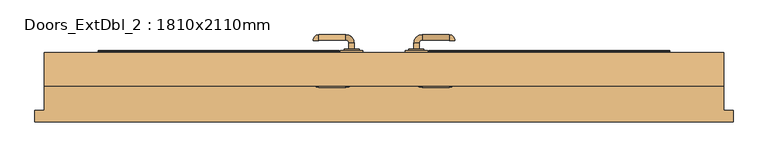
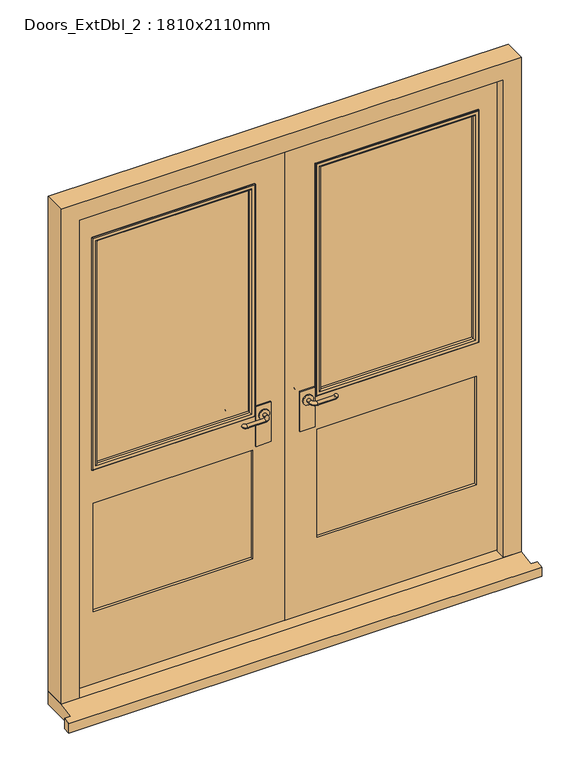
"""IFC4 building model written with IfcOpenShell, lengths in millimetres: door geometry, Doors_ExtDbl_2 : 1810x2110mm."""

from ifc_helpers import new_model, si_unit, point, frame, frame_2d, origin, place, context, project, spatial, polyline, circle_curve, ellipse_curve, trimmed, segment, composite_curve, outline, extrude, faceted_brep, source, transform, mapped, element, save
from ifc_brep_helpers import plane_surface, cylinder_surface, revolved_surface, advanced_brep


def doors_extdbl_2_1810x2110mm_9ab1935a(model_context):
    return source(origin(), model_context, "Body", "SolidModel", [
        extrude(outline(composite_curve([segment(trimmed(circle_curve(frame_2d((950.0, 86.5)), 20.0), [point((950.0, 66.5))], [point((950.0, 106.5))], False, "CARTESIAN"), True, "CONTINUOUS"), segment(trimmed(circle_curve(frame_2d((950.0, 86.5)), 20.0), [point((950.0, 106.5))], [point((950.0, 66.5))], False, "CARTESIAN"), True, "CONTINUOUS")], self_intersect=False)), frame((0.0, 58.4, 0.0), z_axis=(0.0, 1.0, 0.0), x_axis=(0.0, 0.0, 1.0)), (0.0, 0.0, 1.0), 4.5929895),
        advanced_brep(
        [(93.5, 62.9929895, 950.0), (79.5, 62.9929895, 950.0), (93.5, 78.4, 950.0), (79.5, 78.4, 950.0), (101.5, 100.4, 950.0), (101.5, 86.4, 950.0), (173.5, 86.4, 950.0), (173.5, 100.4, 950.0), (174.5, 85.4, 950.0), (188.5, 85.4, 950.0)],
        [
            (0, 1, circle_curve(frame((86.5, 62.9929895, 950.0), z_axis=(0.0, -1.0, 0.0), x_axis=(-1.0, 0.0, 0.0)), 7.0)),
            (1, 0, circle_curve(frame((86.5, 62.9929895, 950.0), z_axis=(0.0, -1.0, 0.0), x_axis=(-1.0, 0.0, 0.0)), 7.0)),
            (0, 2),
            (2, 3, circle_curve(frame((86.5, 78.4, 950.0), z_axis=(0.0, -1.0, 0.0), x_axis=(-1.0, 0.0, 0.0)), 7.0)),
            (3, 1),
            (3, 2, circle_curve(frame((86.5, 78.4, 950.0), z_axis=(0.0, -1.0, 0.0), x_axis=(-1.0, 0.0, 0.0)), 7.0)),
            (4, 3, circle_curve(frame((101.5, 78.4, 950.0), z_axis=(0.0, 0.0, 1.0), x_axis=(-1.0, 0.0, 0.0)), 22.0)),
            (2, 5, circle_curve(frame((101.5, 78.4, 950.0), z_axis=(0.0, 0.0, -1.0), x_axis=(-1.0, 0.0, 0.0)), 8.0)),
            (5, 4, circle_curve(frame((101.5, 93.4, 950.0), z_axis=(-1.0, 0.0, 0.0), x_axis=(0.0, 1.0, 0.0)), 7.0)),
            (4, 5, circle_curve(frame((101.5, 93.4, 950.0), z_axis=(-1.0, 0.0, 0.0), x_axis=(0.0, 1.0, 0.0)), 7.0)),
            (5, 6),
            (6, 7, circle_curve(frame((173.5, 93.4, 950.0), z_axis=(-1.0, 0.0, 0.0), x_axis=(0.0, 1.0, 0.0)), 7.0)),
            (7, 4),
            (7, 6, circle_curve(frame((173.5, 93.4, 950.0), z_axis=(-1.0, 0.0, 0.0), x_axis=(0.0, 1.0, 0.0)), 7.0)),
            (8, 9, circle_curve(frame((181.5, 85.4, 950.0), z_axis=(0.0, -1.0, 0.0), x_axis=(1.0, 0.0, 0.0)), 7.0)),
            (9, 8, circle_curve(frame((181.5, 85.4, 950.0), z_axis=(0.0, -1.0, 0.0), x_axis=(1.0, 0.0, 0.0)), 7.0)),
            (9, 7, circle_curve(frame((173.5, 85.4, 950.0), z_axis=(0.0, 0.0, 1.0), x_axis=(0.0, 1.0, 0.0)), 15.0)),
            (6, 8, circle_curve(frame((173.5, 85.4, 950.0), z_axis=(0.0, 0.0, -1.0), x_axis=(0.0, 1.0, 0.0)), 1.0)),
        ],
        [
            plane_surface(frame((86.5, 62.9929895, 950.0), z_axis=(0.0, -1.0, 0.0), x_axis=(0.0, 0.0, 1.0))),
            cylinder_surface(frame((86.5, 62.9929895, 950.0), z_axis=(0.0, -1.0, 0.0), x_axis=(-1.0, 0.0, 0.0)), 7.0),
            revolved_surface(trimmed(ellipse_curve(frame((86.5, 78.4, 950.0), z_axis=(0.0, -1.0, 0.0), x_axis=(-1.0, 0.0, 0.0)), 7.0, 7.0), [point((93.5, 78.4, 950.0))], [point((79.5, 78.4, 950.0))], True, "CARTESIAN"), (101.5, 78.4, 950.0), (0.0, 0.0, -1.0)),
            revolved_surface(trimmed(ellipse_curve(frame((86.5, 78.4, 950.0), z_axis=(0.0, -1.0, 0.0), x_axis=(-1.0, 0.0, 0.0)), 7.0, 7.0), [point((79.5, 78.4, 950.0))], [point((93.5, 78.4, 950.0))], True, "CARTESIAN"), (101.5, 78.4, 950.0), (0.0, 0.0, -1.0)),
            cylinder_surface(frame((101.5, 93.4, 950.0), z_axis=(-1.0, 0.0, 0.0), x_axis=(0.0, 1.0, 0.0)), 7.0),
            plane_surface(frame((181.5, 85.4, 950.0), z_axis=(0.0, -1.0, 0.0), x_axis=(0.0, 0.0, 1.0))),
            revolved_surface(trimmed(ellipse_curve(frame((173.5, 93.4, 950.0), z_axis=(-1.0, 0.0, 0.0), x_axis=(0.0, 1.0, 0.0)), 7.0, 7.0), [point((173.5, 86.4, 950.0))], [point((173.5, 100.4, 950.0))], True, "CARTESIAN"), (173.5, 85.4, 950.0), (0.0, 0.0, -1.0)),
            revolved_surface(trimmed(ellipse_curve(frame((173.5, 93.4, 950.0), z_axis=(-1.0, 0.0, 0.0), x_axis=(0.0, 1.0, 0.0)), 7.0, 7.0), [point((173.5, 100.4, 950.0))], [point((173.5, 86.4, 950.0))], True, "CARTESIAN"), (173.5, 85.4, 950.0), (0.0, 0.0, -1.0)),
        ],
        [
            (0, [[1, 2]]),
            (1, [[-1, 3, 4, 5]]),
            (1, [[-2, -5, 6, -3]]),
            (2, [[7, -4, 8, 9]]),
            (3, [[-8, -6, -7, 10]]),
            (4, [[-9, 11, 12, 13]]),
            (4, [[-10, -13, 14, -11]]),
            (5, [[15, 16]]),
            (6, [[17, -12, 18, -16]]),
            (7, [[-18, -14, -17, -15]]),
        ],
    ),
        extrude(outline(polyline([(116.5, 52.4), (56.5, 52.4), (56.5, 58.4), (116.5, 58.4), (116.5, 52.4)])), frame((0.0, 0.0, 825.0), z_axis=(0.0, 0.0, 1.0), x_axis=(1.0, 0.0, 0.0)), (0.0, 0.0, 1.0), 165.0),
        extrude(outline(composite_curve([segment(trimmed(circle_curve(frame_2d((950.0, -86.5)), 20.0), [point((950.0, -66.5))], [point((950.0, -106.5))], False, "CARTESIAN"), True, "CONTINUOUS"), segment(trimmed(circle_curve(frame_2d((950.0, -86.5)), 20.0), [point((950.0, -106.5))], [point((950.0, -66.5))], False, "CARTESIAN"), True, "CONTINUOUS")], self_intersect=False)), frame((0.0, 58.4, 0.0), z_axis=(0.0, 1.0, 0.0), x_axis=(0.0, 0.0, 1.0)), (0.0, 0.0, 1.0), 4.5929895),
        advanced_brep(
        [(-93.5, 62.9929895, 950.0), (-79.5, 62.9929895, 950.0), (-79.5, 78.4, 950.0), (-93.5, 78.4, 950.0), (-101.5, 100.4, 950.0), (-101.5, 86.4, 950.0), (-173.5, 100.4, 950.0), (-173.5, 86.4, 950.0), (-174.5, 85.4, 950.0), (-188.5, 85.4, 950.0)],
        [
            (0, 1, circle_curve(frame((-86.5, 62.9929895, 950.0), z_axis=(0.0, -1.0, 0.0), x_axis=(1.0, 0.0, 0.0)), 7.0)),
            (1, 0, circle_curve(frame((-86.5, 62.9929895, 950.0), z_axis=(0.0, -1.0, 0.0), x_axis=(1.0, 0.0, 0.0)), 7.0)),
            (1, 2),
            (2, 3, circle_curve(frame((-86.5, 78.4, 950.0), z_axis=(0.0, -1.0, 0.0), x_axis=(1.0, 0.0, 0.0)), 7.0)),
            (3, 0),
            (3, 2, circle_curve(frame((-86.5, 78.4, 950.0), z_axis=(0.0, -1.0, 0.0), x_axis=(1.0, 0.0, 0.0)), 7.0)),
            (4, 5, circle_curve(frame((-101.5, 93.4, 950.0), z_axis=(1.0, 0.0, 0.0), x_axis=(0.0, 1.0, 0.0)), 7.0)),
            (5, 3, circle_curve(frame((-101.5, 78.4, 950.0), z_axis=(0.0, 0.0, -1.0), x_axis=(1.0, 0.0, 0.0)), 8.0)),
            (2, 4, circle_curve(frame((-101.5, 78.4, 950.0), z_axis=(0.0, 0.0, 1.0), x_axis=(1.0, 0.0, 0.0)), 22.0)),
            (5, 4, circle_curve(frame((-101.5, 93.4, 950.0), z_axis=(1.0, 0.0, 0.0), x_axis=(0.0, 1.0, 0.0)), 7.0)),
            (4, 6),
            (6, 7, circle_curve(frame((-173.5, 93.4, 950.0), z_axis=(1.0, 0.0, 0.0), x_axis=(0.0, 1.0, 0.0)), 7.0)),
            (7, 5),
            (7, 6, circle_curve(frame((-173.5, 93.4, 950.0), z_axis=(1.0, 0.0, 0.0), x_axis=(0.0, 1.0, 0.0)), 7.0)),
            (8, 9, circle_curve(frame((-181.5, 85.4, 950.0), z_axis=(0.0, -1.0, 0.0), x_axis=(-1.0, 0.0, 0.0)), 7.0)),
            (9, 8, circle_curve(frame((-181.5, 85.4, 950.0), z_axis=(0.0, -1.0, 0.0), x_axis=(-1.0, 0.0, 0.0)), 7.0)),
            (8, 7, circle_curve(frame((-173.5, 85.4, 950.0), z_axis=(0.0, 0.0, -1.0), x_axis=(0.0, 1.0, 0.0)), 1.0)),
            (6, 9, circle_curve(frame((-173.5, 85.4, 950.0), z_axis=(0.0, 0.0, 1.0), x_axis=(0.0, 1.0, 0.0)), 15.0)),
        ],
        [
            plane_surface(frame((-86.5, 62.9929895, 950.0), z_axis=(0.0, -1.0, 0.0), x_axis=(0.0, 0.0, 1.0))),
            cylinder_surface(frame((-86.5, 62.9929895, 950.0), z_axis=(0.0, -1.0, 0.0), x_axis=(1.0, 0.0, 0.0)), 7.0),
            revolved_surface(trimmed(ellipse_curve(frame((-86.5, 78.4, 950.0), z_axis=(0.0, 1.0, 0.0), x_axis=(1.0, 0.0, 0.0)), 7.0, 7.0), [point((-93.5, 78.4, 950.0))], [point((-79.5, 78.4, 950.0))], True, "CARTESIAN"), (-101.5, 78.4, 950.0), (0.0, 0.0, -1.0)),
            revolved_surface(trimmed(ellipse_curve(frame((-86.5, 78.4, 950.0), z_axis=(0.0, 1.0, 0.0), x_axis=(1.0, 0.0, 0.0)), 7.0, 7.0), [point((-79.5, 78.4, 950.0))], [point((-93.5, 78.4, 950.0))], True, "CARTESIAN"), (-101.5, 78.4, 950.0), (0.0, 0.0, -1.0)),
            cylinder_surface(frame((-101.5, 93.4, 950.0), z_axis=(1.0, 0.0, 0.0), x_axis=(0.0, 1.0, 0.0)), 7.0),
            plane_surface(frame((-181.5, 85.4, 950.0), z_axis=(0.0, -1.0, 0.0), x_axis=(0.0, 0.0, 1.0))),
            revolved_surface(trimmed(ellipse_curve(frame((-173.5, 93.4, 950.0), z_axis=(-1.0, 0.0, 0.0), x_axis=(0.0, 1.0, 0.0)), 7.0, 7.0), [point((-173.5, 86.4, 950.0))], [point((-173.5, 100.4, 950.0))], True, "CARTESIAN"), (-173.5, 85.4, 950.0), (0.0, 0.0, -1.0)),
            revolved_surface(trimmed(ellipse_curve(frame((-173.5, 93.4, 950.0), z_axis=(-1.0, 0.0, 0.0), x_axis=(0.0, 1.0, 0.0)), 7.0, 7.0), [point((-173.5, 100.4, 950.0))], [point((-173.5, 86.4, 950.0))], True, "CARTESIAN"), (-173.5, 85.4, 950.0), (0.0, 0.0, -1.0)),
        ],
        [
            (0, [[1, 2]]),
            (1, [[3, 4, 5, -2]]),
            (1, [[-5, 6, -3, -1]]),
            (2, [[7, 8, -4, 9]]),
            (3, [[10, -9, -6, -8]]),
            (4, [[11, 12, 13, -7]]),
            (4, [[-13, 14, -11, -10]]),
            (5, [[15, 16]]),
            (6, [[-15, 17, -12, 18]]),
            (7, [[-16, -18, -14, -17]]),
        ],
    ),
        extrude(outline(polyline([(-116.5, 52.4), (-116.5, 58.4), (-56.5, 58.4), (-56.5, 52.4), (-116.5, 52.4)])), frame((0.0, 0.0, 825.0), z_axis=(0.0, 0.0, 1.0), x_axis=(1.0, 0.0, 0.0)), (0.0, 0.0, 1.0), 165.0),
        extrude(outline(composite_curve([segment(trimmed(circle_curve(frame_2d((950.0, -86.5)), 20.0), [point((950.0, -66.5))], [point((950.0, -106.5))], False, "CARTESIAN"), True, "CONTINUOUS"), segment(trimmed(circle_curve(frame_2d((950.0, -86.5)), 20.0), [point((950.0, -106.5))], [point((950.0, -66.5))], False, "CARTESIAN"), True, "CONTINUOUS")], self_intersect=False)), frame((0.0, -2.1929895, 0.0), z_axis=(0.0, 1.0, 0.0), x_axis=(0.0, 0.0, 1.0)), (0.0, 0.0, 1.0), 4.5929895),
        advanced_brep(
        [(-93.5, -2.1929895, 950.0), (-79.5, -2.1929895, 950.0), (-93.5, -17.6, 950.0), (-79.5, -17.6, 950.0), (-101.5, -39.6, 950.0), (-101.5, -25.6, 950.0), (-173.5, -25.6, 950.0), (-173.5, -39.6, 950.0), (-174.5, -24.6, 950.0), (-188.5, -24.6, 950.0)],
        [
            (0, 1, circle_curve(frame((-86.5, -2.1929895, 950.0), z_axis=(0.0, 1.0, 0.0), x_axis=(1.0, 0.0, 0.0)), 7.0)),
            (1, 0, circle_curve(frame((-86.5, -2.1929895, 950.0), z_axis=(0.0, 1.0, 0.0), x_axis=(1.0, 0.0, 0.0)), 7.0)),
            (0, 2),
            (2, 3, circle_curve(frame((-86.5, -17.6, 950.0), z_axis=(0.0, 1.0, 0.0), x_axis=(1.0, 0.0, 0.0)), 7.0)),
            (3, 1),
            (3, 2, circle_curve(frame((-86.5, -17.6, 950.0), z_axis=(0.0, 1.0, 0.0), x_axis=(1.0, 0.0, 0.0)), 7.0)),
            (4, 3, circle_curve(frame((-101.5, -17.6, 950.0), z_axis=(0.0, 0.0, 1.0), x_axis=(1.0, 0.0, 0.0)), 22.0)),
            (2, 5, circle_curve(frame((-101.5, -17.6, 950.0), z_axis=(0.0, 0.0, -1.0), x_axis=(1.0, 0.0, 0.0)), 8.0)),
            (5, 4, circle_curve(frame((-101.5, -32.6, 950.0), z_axis=(1.0, 0.0, 0.0), x_axis=(0.0, -1.0, 0.0)), 7.0)),
            (4, 5, circle_curve(frame((-101.5, -32.6, 950.0), z_axis=(1.0, 0.0, 0.0), x_axis=(0.0, -1.0, 0.0)), 7.0)),
            (5, 6),
            (6, 7, circle_curve(frame((-173.5, -32.6, 950.0), z_axis=(1.0, 0.0, 0.0), x_axis=(0.0, -1.0, 0.0)), 7.0)),
            (7, 4),
            (7, 6, circle_curve(frame((-173.5, -32.6, 950.0), z_axis=(1.0, 0.0, 0.0), x_axis=(0.0, -1.0, 0.0)), 7.0)),
            (8, 9, circle_curve(frame((-181.5, -24.6, 950.0), z_axis=(0.0, 1.0, 0.0), x_axis=(-1.0, 0.0, 0.0)), 7.0)),
            (9, 8, circle_curve(frame((-181.5, -24.6, 950.0), z_axis=(0.0, 1.0, 0.0), x_axis=(-1.0, 0.0, 0.0)), 7.0)),
            (9, 7, circle_curve(frame((-173.5, -24.6, 950.0), z_axis=(0.0, 0.0, 1.0), x_axis=(0.0, -1.0, 0.0)), 15.0)),
            (6, 8, circle_curve(frame((-173.5, -24.6, 950.0), z_axis=(0.0, 0.0, -1.0), x_axis=(0.0, -1.0, 0.0)), 1.0)),
        ],
        [
            plane_surface(frame((-86.5, -2.1929895, 950.0), z_axis=(0.0, 1.0, 0.0), x_axis=(0.0, 0.0, 1.0))),
            cylinder_surface(frame((-86.5, -2.1929895, 950.0), z_axis=(0.0, 1.0, 0.0), x_axis=(1.0, 0.0, 0.0)), 7.0),
            revolved_surface(trimmed(ellipse_curve(frame((-86.5, -17.6, 950.0), z_axis=(0.0, 1.0, 0.0), x_axis=(1.0, 0.0, 0.0)), 7.0, 7.0), [point((-93.5, -17.6, 950.0))], [point((-79.5, -17.6, 950.0))], True, "CARTESIAN"), (-101.5, -17.6, 950.0), (0.0, 0.0, -1.0)),
            revolved_surface(trimmed(ellipse_curve(frame((-86.5, -17.6, 950.0), z_axis=(0.0, 1.0, 0.0), x_axis=(1.0, 0.0, 0.0)), 7.0, 7.0), [point((-79.5, -17.6, 950.0))], [point((-93.5, -17.6, 950.0))], True, "CARTESIAN"), (-101.5, -17.6, 950.0), (0.0, 0.0, -1.0)),
            cylinder_surface(frame((-101.5, -32.6, 950.0), z_axis=(1.0, 0.0, 0.0), x_axis=(0.0, -1.0, 0.0)), 7.0),
            plane_surface(frame((-181.5, -24.6, 950.0), z_axis=(0.0, 1.0, 0.0), x_axis=(0.0, 0.0, 1.0))),
            revolved_surface(trimmed(ellipse_curve(frame((-173.5, -32.6, 950.0), z_axis=(1.0, 0.0, 0.0), x_axis=(0.0, -1.0, 0.0)), 7.0, 7.0), [point((-173.5, -25.6, 950.0))], [point((-173.5, -39.6, 950.0))], True, "CARTESIAN"), (-173.5, -24.6, 950.0), (0.0, 0.0, -1.0)),
            revolved_surface(trimmed(ellipse_curve(frame((-173.5, -32.6, 950.0), z_axis=(1.0, 0.0, 0.0), x_axis=(0.0, -1.0, 0.0)), 7.0, 7.0), [point((-173.5, -39.6, 950.0))], [point((-173.5, -25.6, 950.0))], True, "CARTESIAN"), (-173.5, -24.6, 950.0), (0.0, 0.0, -1.0)),
        ],
        [
            (0, [[1, 2]]),
            (1, [[-1, 3, 4, 5]]),
            (1, [[-2, -5, 6, -3]]),
            (2, [[7, -4, 8, 9]]),
            (3, [[-8, -6, -7, 10]]),
            (4, [[-9, 11, 12, 13]]),
            (4, [[-10, -13, 14, -11]]),
            (5, [[15, 16]]),
            (6, [[17, -12, 18, -16]]),
            (7, [[-18, -14, -17, -15]]),
        ],
    ),
        extrude(outline(polyline([(-116.5, 8.4), (-56.5, 8.4), (-56.5, 2.4), (-116.5, 2.4), (-116.5, 8.4)])), frame((0.0, 0.0, 825.0), z_axis=(0.0, 0.0, 1.0), x_axis=(1.0, 0.0, 0.0)), (0.0, 0.0, 1.0), 165.0),
        extrude(outline(composite_curve([segment(trimmed(circle_curve(frame_2d((950.0, 86.5)), 20.0), [point((950.0, 66.5))], [point((950.0, 106.5))], False, "CARTESIAN"), True, "CONTINUOUS"), segment(trimmed(circle_curve(frame_2d((950.0, 86.5)), 20.0), [point((950.0, 106.5))], [point((950.0, 66.5))], False, "CARTESIAN"), True, "CONTINUOUS")], self_intersect=False)), frame((0.0, -2.1929895, 0.0), z_axis=(0.0, 1.0, 0.0), x_axis=(0.0, 0.0, 1.0)), (0.0, 0.0, 1.0), 4.5929895),
        advanced_brep(
        [(93.5, -2.1929895, 950.0), (79.5, -2.1929895, 950.0), (79.5, -17.6, 950.0), (93.5, -17.6, 950.0), (101.5, -39.6, 950.0), (101.5, -25.6, 950.0), (173.5, -39.6, 950.0), (173.5, -25.6, 950.0), (174.5, -24.6, 950.0), (188.5, -24.6, 950.0)],
        [
            (0, 1, circle_curve(frame((86.5, -2.1929895, 950.0), z_axis=(0.0, 1.0, 0.0), x_axis=(-1.0, 0.0, 0.0)), 7.0)),
            (1, 0, circle_curve(frame((86.5, -2.1929895, 950.0), z_axis=(0.0, 1.0, 0.0), x_axis=(-1.0, 0.0, 0.0)), 7.0)),
            (1, 2),
            (2, 3, circle_curve(frame((86.5, -17.6, 950.0), z_axis=(0.0, 1.0, 0.0), x_axis=(-1.0, 0.0, 0.0)), 7.0)),
            (3, 0),
            (3, 2, circle_curve(frame((86.5, -17.6, 950.0), z_axis=(0.0, 1.0, 0.0), x_axis=(-1.0, 0.0, 0.0)), 7.0)),
            (4, 5, circle_curve(frame((101.5, -32.6, 950.0), z_axis=(-1.0, 0.0, 0.0), x_axis=(0.0, -1.0, 0.0)), 7.0)),
            (5, 3, circle_curve(frame((101.5, -17.6, 950.0), z_axis=(0.0, 0.0, -1.0), x_axis=(-1.0, 0.0, 0.0)), 8.0)),
            (2, 4, circle_curve(frame((101.5, -17.6, 950.0), z_axis=(0.0, 0.0, 1.0), x_axis=(-1.0, 0.0, 0.0)), 22.0)),
            (5, 4, circle_curve(frame((101.5, -32.6, 950.0), z_axis=(-1.0, 0.0, 0.0), x_axis=(0.0, -1.0, 0.0)), 7.0)),
            (4, 6),
            (6, 7, circle_curve(frame((173.5, -32.6, 950.0), z_axis=(-1.0, 0.0, 0.0), x_axis=(0.0, -1.0, 0.0)), 7.0)),
            (7, 5),
            (7, 6, circle_curve(frame((173.5, -32.6, 950.0), z_axis=(-1.0, 0.0, 0.0), x_axis=(0.0, -1.0, 0.0)), 7.0)),
            (8, 9, circle_curve(frame((181.5, -24.6, 950.0), z_axis=(0.0, 1.0, 0.0), x_axis=(1.0, 0.0, 0.0)), 7.0)),
            (9, 8, circle_curve(frame((181.5, -24.6, 950.0), z_axis=(0.0, 1.0, 0.0), x_axis=(1.0, 0.0, 0.0)), 7.0)),
            (8, 7, circle_curve(frame((173.5, -24.6, 950.0), z_axis=(0.0, 0.0, -1.0), x_axis=(0.0, -1.0, 0.0)), 1.0)),
            (6, 9, circle_curve(frame((173.5, -24.6, 950.0), z_axis=(0.0, 0.0, 1.0), x_axis=(0.0, -1.0, 0.0)), 15.0)),
        ],
        [
            plane_surface(frame((86.5, -2.1929895, 950.0), z_axis=(0.0, 1.0, 0.0), x_axis=(0.0, 0.0, 1.0))),
            cylinder_surface(frame((86.5, -2.1929895, 950.0), z_axis=(0.0, 1.0, 0.0), x_axis=(-1.0, 0.0, 0.0)), 7.0),
            revolved_surface(trimmed(ellipse_curve(frame((86.5, -17.6, 950.0), z_axis=(0.0, -1.0, 0.0), x_axis=(-1.0, 0.0, 0.0)), 7.0, 7.0), [point((93.5, -17.6, 950.0))], [point((79.5, -17.6, 950.0))], True, "CARTESIAN"), (101.5, -17.6, 950.0), (0.0, 0.0, -1.0)),
            revolved_surface(trimmed(ellipse_curve(frame((86.5, -17.6, 950.0), z_axis=(0.0, -1.0, 0.0), x_axis=(-1.0, 0.0, 0.0)), 7.0, 7.0), [point((79.5, -17.6, 950.0))], [point((93.5, -17.6, 950.0))], True, "CARTESIAN"), (101.5, -17.6, 950.0), (0.0, 0.0, -1.0)),
            cylinder_surface(frame((101.5, -32.6, 950.0), z_axis=(-1.0, 0.0, 0.0), x_axis=(0.0, -1.0, 0.0)), 7.0),
            plane_surface(frame((181.5, -24.6, 950.0), z_axis=(0.0, 1.0, 0.0), x_axis=(0.0, 0.0, 1.0))),
            revolved_surface(trimmed(ellipse_curve(frame((173.5, -32.6, 950.0), z_axis=(1.0, 0.0, 0.0), x_axis=(0.0, -1.0, 0.0)), 7.0, 7.0), [point((173.5, -25.6, 950.0))], [point((173.5, -39.6, 950.0))], True, "CARTESIAN"), (173.5, -24.6, 950.0), (0.0, 0.0, -1.0)),
            revolved_surface(trimmed(ellipse_curve(frame((173.5, -32.6, 950.0), z_axis=(1.0, 0.0, 0.0), x_axis=(0.0, -1.0, 0.0)), 7.0, 7.0), [point((173.5, -39.6, 950.0))], [point((173.5, -25.6, 950.0))], True, "CARTESIAN"), (173.5, -24.6, 950.0), (0.0, 0.0, -1.0)),
        ],
        [
            (0, [[1, 2]]),
            (1, [[3, 4, 5, -2]]),
            (1, [[-5, 6, -3, -1]]),
            (2, [[7, 8, -4, 9]]),
            (3, [[10, -9, -6, -8]]),
            (4, [[11, 12, 13, -7]]),
            (4, [[-13, 14, -11, -10]]),
            (5, [[15, 16]]),
            (6, [[-15, 17, -12, 18]]),
            (7, [[-16, -18, -14, -17]]),
        ],
    ),
        extrude(outline(polyline([(116.5, 8.4), (116.5, 2.4), (56.5, 2.4), (56.5, 8.4), (116.5, 8.4)])), frame((0.0, 0.0, 825.0), z_axis=(0.0, 0.0, 1.0), x_axis=(1.0, 0.0, 0.0)), (0.0, 0.0, 1.0), 165.0),
        faceted_brep([(834.5, -36.6, 54.5), (834.5, 5.4, 54.5), (856.5, 5.4, 54.5), (856.5, 52.4, 54.5), (905.0, 52.4, 54.5), (905.0, -36.6, 54.5), (905.0, -36.6, 2110.0), (-905.0, -36.6, 2110.0), (-905.0, -36.6, 54.5), (-834.5, -36.6, 54.5), (-834.5, -36.6, 2039.5), (834.5, -36.6, 2039.5), (905.0, 52.4, 2110.0), (856.5, 52.4, 2061.5), (-856.5, 52.4, 2061.5), (-856.5, 52.4, 54.5), (-905.0, 52.4, 54.5), (-905.0, 52.4, 2110.0), (856.5, 5.4, 2061.5), (834.5, 5.4, 2039.5), (-834.5, 5.4, 2039.5), (-834.5, 5.4, 54.5), (-856.5, 5.4, 54.5), (-856.5, 5.4, 2061.5)], [[[0, 1, 2, 3, 4, 5]], [[5, 6, 7, 8, 9, 10, 11, 0]], [[4, 12, 6, 5]], [[3, 13, 14, 15, 16, 17, 12, 4]], [[2, 18, 13, 3]], [[1, 19, 20, 21, 22, 23, 18, 2]], [[0, 11, 19, 1]], [[10, 9, 21, 20]], [[9, 8, 16, 15, 22, 21]], [[17, 16, 8, 7]], [[23, 22, 15, 14]], [[12, 17, 7, 6]], [[18, 23, 14, 13]], [[11, 10, 20, 19]]]),
        extrude(outline(polyline([(58.5, 853.5), (2058.5, 853.5), (2058.5, 1.5), (58.5, 1.5), (58.5, 853.5)]), holes=[polyline([(1908.5, 753.5), (958.5, 753.5), (958.5, 126.5), (1908.5, 126.5), (1908.5, 753.5)]), polyline([(808.5, 126.5), (808.5, 753.5), (358.5, 753.5), (358.5, 126.5), (808.5, 126.5)])]), frame((0.0, 8.4, 0.0), z_axis=(0.0, 1.0, 0.0), x_axis=(0.0, 0.0, 1.0)), (0.0, 0.0, 1.0), 44.0),
        extrude(outline(polyline([(58.5, -853.5), (58.5, -1.5), (2058.5, -1.5), (2058.5, -853.5), (58.5, -853.5)]), holes=[polyline([(1908.5, -126.5), (958.5, -126.5), (958.5, -753.5), (1908.5, -753.5), (1908.5, -126.5)]), polyline([(808.5, -753.5), (808.5, -126.5), (358.5, -126.5), (358.5, -753.5), (808.5, -753.5)])]), frame((0.0, 8.4, 0.0), z_axis=(0.0, 1.0, 0.0), x_axis=(0.0, 0.0, 1.0)), (0.0, 0.0, 1.0), 44.0),
        faceted_brep([(930.0, -131.6, 0.0), (930.0, -101.6, 0.0), (930.0, -101.6, 43.6174415), (930.0, -131.6, 38.5947221), (-930.0, -131.6, 38.5947221), (-930.0, -101.6, 43.6174415), (-930.0, -101.6, 0.0), (-930.0, -131.6, 0.0), (-905.0, -101.6, 0.0), (-905.0, 52.4, 0.0), (905.0, 52.4, 0.0), (905.0, -101.6, 0.0), (905.0, -101.6, 43.6174415), (905.0, -36.6, 54.5), (-905.0, -36.6, 54.5), (-905.0, -101.6, 43.6174415), (905.0, 52.4, 54.5), (-905.0, 52.4, 54.5)], [[[0, 1, 2, 3]], [[4, 5, 6, 7]], [[7, 6, 8, 9, 10, 11, 1, 0]], [[3, 4, 7, 0]], [[3, 2, 12, 13, 14, 15, 5, 4]], [[14, 13, 16, 17]], [[17, 16, 10, 9]], [[15, 14, 17, 9, 8]], [[8, 6, 5, 15]], [[11, 10, 16, 13, 12]], [[12, 2, 1, 11]]]),
        extrude(outline(polyline([(126.5, 18.4), (126.5, 42.4), (751.9390207, 42.4), (751.9390207, 18.4), (126.5, 18.4)])), frame((0.0, 0.0, 958.5), z_axis=(0.0, 0.0, 1.0), x_axis=(1.0, 0.0, 0.0)), (0.0, 0.0, 1.0), 950.0),
        extrude(outline(polyline([(-753.5, 18.4), (-753.5, 42.4), (-126.5, 42.4), (-126.5, 18.4), (-753.5, 18.4)])), frame((0.0, 0.0, 958.5), z_axis=(0.0, 0.0, 1.0), x_axis=(1.0, 0.0, 0.0)), (0.0, 0.0, 1.0), 950.0),
        extrude(outline(polyline([(753.5, 42.4), (753.5, 18.4), (126.5, 18.4), (126.5, 42.4), (753.5, 42.4)])), frame((0.0, 0.0, 358.5), z_axis=(0.0, 0.0, 1.0), x_axis=(1.0, 0.0, 0.0)), (0.0, 0.0, 1.0), 450.0),
        extrude(outline(polyline([(-126.5, 42.4), (-126.5, 18.4), (-753.5, 18.4), (-753.5, 42.4), (-126.5, 42.4)])), frame((0.0, 0.0, 358.5), z_axis=(0.0, 0.0, 1.0), x_axis=(1.0, 0.0, 0.0)), (0.0, 0.0, 1.0), 450.0),
        advanced_brep(
        [(118.5, 4.4, 950.5), (118.5, 4.4, 1916.5), (118.5, 8.4, 1916.5), (118.5, 8.4, 950.5), (120.5, 2.4, 952.5), (120.5, 2.4, 1914.5), (138.5, 7.4, 970.5), (138.5, 7.4, 1896.5), (133.5, 2.4, 1901.5), (133.5, 2.4, 965.5), (138.5, 18.4, 970.5), (138.5, 18.4, 1896.5), (126.5, 8.4, 958.5), (126.5, 8.4, 1908.5), (126.5, 18.4, 1908.5), (126.5, 18.4, 958.5), (761.5, 4.4, 1916.5), (761.5, 8.4, 1916.5), (759.5, 2.4, 1914.5), (741.5, 7.4, 1896.5), (746.5, 2.4, 1901.5), (741.5, 18.4, 1896.5), (753.5, 8.4, 1908.5), (753.5, 18.4, 1908.5), (761.5, 4.4, 950.5), (761.5, 8.4, 950.5), (759.5, 2.4, 952.5), (741.5, 7.4, 970.5), (746.5, 2.4, 965.5), (741.5, 18.4, 970.5), (753.5, 8.4, 958.5), (753.5, 18.4, 958.5)],
        [
            (0, 1),
            (1, 2),
            (2, 3),
            (3, 0),
            (4, 5),
            (5, 1, ellipse_curve(frame((120.5, 4.4, 1914.5), z_axis=(-0.7071067811865476, 0.0, -0.7071067811865474), x_axis=(0.7071067811865472, 0.0, -0.7071067811865478)), 2.8284271, 2.0)),
            (0, 4, ellipse_curve(frame((120.5, 4.4, 952.5), z_axis=(-0.7071067811865474, 0.0, 0.7071067811865476), x_axis=(-0.7071067811865475, 0.0, -0.7071067811865475)), 2.8284271, 2.0)),
            (6, 7),
            (7, 8, ellipse_curve(frame((133.5, 7.4, 1901.5), z_axis=(-0.7071067811865476, 0.0, -0.7071067811865474), x_axis=(0.7071067811865472, 0.0, -0.7071067811865478)), 7.0710678, 5.0)),
            (8, 9),
            (9, 6, ellipse_curve(frame((133.5, 7.4, 965.5), z_axis=(-0.7071067811865474, 0.0, 0.7071067811865476), x_axis=(-0.7071067811865475, 0.0, -0.7071067811865475)), 7.0710678, 5.0)),
            (10, 11),
            (11, 7),
            (6, 10),
            (12, 13),
            (13, 14),
            (14, 15),
            (15, 12),
            (1, 16),
            (16, 17),
            (17, 2),
            (5, 18),
            (18, 16, ellipse_curve(frame((759.5, 4.4, 1914.5), z_axis=(-0.7071067811865474, 0.0, 0.7071067811865477), x_axis=(-0.7071067811865477, 0.0, -0.7071067811865474)), 2.8284271, 2.0)),
            (7, 19),
            (19, 20, ellipse_curve(frame((746.5, 7.4, 1901.5), z_axis=(-0.7071067811865474, 0.0, 0.7071067811865477), x_axis=(-0.7071067811865477, 0.0, -0.7071067811865474)), 7.0710678, 5.0)),
            (20, 8),
            (11, 21),
            (21, 19),
            (13, 22),
            (22, 23),
            (23, 14),
            (16, 24),
            (24, 25),
            (25, 17),
            (18, 26),
            (26, 24, ellipse_curve(frame((759.5, 4.4, 952.5), z_axis=(0.7071067811865478, 0.0, 0.7071067811865472), x_axis=(-0.7071067811865471, 0.0, 0.7071067811865478)), 2.8284271, 2.0)),
            (19, 27),
            (27, 28, ellipse_curve(frame((746.5, 7.4, 965.5), z_axis=(0.7071067811865478, 0.0, 0.7071067811865472), x_axis=(-0.7071067811865471, 0.0, 0.7071067811865478)), 7.0710678, 5.0)),
            (28, 20),
            (21, 29),
            (29, 27),
            (22, 30),
            (30, 31),
            (31, 23),
            (24, 0),
            (3, 25),
            (26, 4),
            (28, 9),
            (27, 6),
            (29, 10),
            (31, 15),
            (30, 12),
        ],
        [
            plane_surface(frame((118.5, 8.4, 950.5), z_axis=(-1.0, 0.0, 0.0), x_axis=(0.0, 0.0, 1.0))),
            cylinder_surface(frame((120.5, 4.4, 958.5), z_axis=(0.0, 0.0, -1.0), x_axis=(-1.0, 0.0, 0.0)), 2.0),
            cylinder_surface(frame((133.5, 7.4, 958.5), z_axis=(0.0, 0.0, -1.0), x_axis=(-1.0, 0.0, 0.0)), 5.0),
            plane_surface(frame((138.5, 7.4, 970.5), z_axis=(1.0, 0.0, 0.0), x_axis=(0.0, 0.0, 1.0))),
            plane_surface(frame((126.5, 18.4, 958.5), z_axis=(-1.0, 0.0, 0.0), x_axis=(0.0, 0.0, 1.0))),
            plane_surface(frame((118.5, 8.4, 1916.5), z_axis=(0.0, 0.0, 1.0), x_axis=(1.0, 0.0, 0.0))),
            cylinder_surface(frame((126.5, 4.4, 1914.5), z_axis=(-1.0, 0.0, 0.0), x_axis=(0.0, 0.0, 1.0)), 2.0),
            cylinder_surface(frame((126.5, 7.4, 1901.5), z_axis=(-1.0, 0.0, 0.0), x_axis=(0.0, 0.0, 1.0)), 5.0),
            plane_surface(frame((138.5, 7.4, 1896.5), z_axis=(0.0, 0.0, -1.0), x_axis=(1.0, 0.0, 0.0))),
            plane_surface(frame((126.5, 18.4, 1908.5), z_axis=(0.0, 0.0, 1.0), x_axis=(1.0, 0.0, 0.0))),
            plane_surface(frame((761.5, 8.4, 1916.5), z_axis=(1.0, 0.0, 0.0), x_axis=(0.0, 0.0, -1.0))),
            cylinder_surface(frame((759.5, 4.4, 1908.5), z_axis=(0.0, 0.0, 1.0), x_axis=(1.0, 0.0, 0.0)), 2.0),
            cylinder_surface(frame((746.5, 7.4, 1908.5), z_axis=(0.0, 0.0, 1.0), x_axis=(1.0, 0.0, 0.0)), 5.0),
            plane_surface(frame((741.5, 7.4, 1896.5), z_axis=(-1.0, 0.0, 0.0), x_axis=(0.0, 0.0, -1.0))),
            plane_surface(frame((753.5, 18.4, 1908.5), z_axis=(1.0, 0.0, 0.0), x_axis=(0.0, 0.0, -1.0))),
            plane_surface(frame((761.5, 8.4, 950.5), z_axis=(0.0, 0.0, -1.0), x_axis=(-1.0, 0.0, 0.0))),
            cylinder_surface(frame((753.5, 4.4, 952.5), z_axis=(1.0, 0.0, 0.0), x_axis=(0.0, 0.0, -1.0)), 2.0),
            plane_surface(frame((759.5, 2.4, 952.5), z_axis=(0.0, -1.0, 0.0), x_axis=(-1.0, 0.0, 0.0))),
            cylinder_surface(frame((753.5, 7.4, 965.5), z_axis=(1.0, 0.0, 0.0), x_axis=(0.0, 0.0, -1.0)), 5.0),
            plane_surface(frame((741.5, 7.4, 970.5), z_axis=(0.0, 0.0, 1.0), x_axis=(-1.0, 0.0, 0.0))),
            plane_surface(frame((741.5, 18.4, 970.5), z_axis=(0.0, 1.0, 0.0), x_axis=(-1.0, 0.0, 0.0))),
            plane_surface(frame((753.5, 18.4, 958.5), z_axis=(0.0, 0.0, -1.0), x_axis=(-1.0, 0.0, 0.0))),
            plane_surface(frame((753.5, 8.4, 958.5), z_axis=(0.0, 1.0, 0.0), x_axis=(-1.0, 0.0, 0.0))),
        ],
        [
            (0, [[1, 2, 3, 4]]),
            (1, [[5, 6, -1, 7]]),
            (2, [[8, 9, 10, 11]]),
            (3, [[12, 13, -8, 14]]),
            (4, [[15, 16, 17, 18]]),
            (5, [[19, 20, 21, -2]]),
            (6, [[22, 23, -19, -6]]),
            (7, [[24, 25, 26, -9]]),
            (8, [[27, 28, -24, -13]]),
            (9, [[29, 30, 31, -16]]),
            (10, [[32, 33, 34, -20]]),
            (11, [[35, 36, -32, -23]]),
            (12, [[37, 38, 39, -25]]),
            (13, [[40, 41, -37, -28]]),
            (14, [[42, 43, 44, -30]]),
            (15, [[45, -4, 46, -33]]),
            (16, [[47, -7, -45, -36]]),
            (17, [[-5, -47, -35, -22], [-10, -26, -39, 48]]),
            (18, [[49, -11, -48, -38]]),
            (19, [[50, -14, -49, -41]]),
            (20, [[-17, -31, -44, 51], [-12, -50, -40, -27]]),
            (21, [[52, -18, -51, -43]]),
            (22, [[-3, -21, -34, -46], [-15, -52, -42, -29]]),
        ],
    ),
        advanced_brep(
        [(753.5, 42.4, 1908.5), (753.5, 42.4, 958.5), (753.5, 52.4, 958.5), (753.5, 52.4, 1908.5), (741.5, 53.4, 1896.5), (741.5, 53.4, 970.5), (741.5, 42.4, 970.5), (741.5, 42.4, 1896.5), (746.5, 58.4, 1901.5), (746.5, 58.4, 965.5), (761.5, 56.4, 1916.5), (761.5, 56.4, 950.5), (759.5, 58.4, 952.5), (759.5, 58.4, 1914.5), (761.5, 52.4, 1916.5), (761.5, 52.4, 950.5), (126.5, 42.4, 958.5), (126.5, 52.4, 958.5), (138.5, 53.4, 970.5), (138.5, 42.4, 970.5), (133.5, 58.4, 965.5), (118.5, 56.4, 950.5), (120.5, 58.4, 952.5), (118.5, 52.4, 950.5), (126.5, 42.4, 1908.5), (126.5, 52.4, 1908.5), (138.5, 53.4, 1896.5), (138.5, 42.4, 1896.5), (133.5, 58.4, 1901.5), (118.5, 56.4, 1916.5), (120.5, 58.4, 1914.5), (118.5, 52.4, 1916.5)],
        [
            (0, 1),
            (1, 2),
            (2, 3),
            (3, 0),
            (4, 5),
            (5, 6),
            (6, 7),
            (7, 4),
            (8, 9),
            (9, 5, ellipse_curve(frame((746.5, 53.4, 965.5), z_axis=(0.7071067811865429, 0.0, 0.707106781186552), x_axis=(-0.7071067811865519, 0.0, 0.707106781186543)), 7.0710678, 5.0)),
            (4, 8, ellipse_curve(frame((746.5, 53.4, 1901.5), z_axis=(0.707106781186552, 0.0, -0.7071067811865429), x_axis=(0.7071067811865428, 0.0, 0.7071067811865521)), 7.0710678, 5.0)),
            (10, 11),
            (11, 12, ellipse_curve(frame((759.5, 56.4, 952.5), z_axis=(0.7071067811865429, 0.0, 0.707106781186552), x_axis=(-0.7071067811865519, 0.0, 0.707106781186543)), 2.8284271, 2.0)),
            (12, 13),
            (13, 10, ellipse_curve(frame((759.5, 56.4, 1914.5), z_axis=(0.707106781186552, 0.0, -0.7071067811865429), x_axis=(0.7071067811865428, 0.0, 0.7071067811865521)), 2.8284271, 2.0)),
            (14, 15),
            (15, 11),
            (10, 14),
            (1, 16),
            (16, 17),
            (17, 2),
            (5, 18),
            (18, 19),
            (19, 6),
            (9, 20),
            (20, 18, ellipse_curve(frame((133.5, 53.4, 965.5), z_axis=(0.707106781186552, 0.0, -0.7071067811865431), x_axis=(0.7071067811865429, 0.0, 0.7071067811865521)), 7.0710678, 5.0)),
            (11, 21),
            (21, 22, ellipse_curve(frame((120.5, 56.4, 952.5), z_axis=(0.707106781186552, 0.0, -0.7071067811865431), x_axis=(0.7071067811865429, 0.0, 0.7071067811865521)), 2.8284271, 2.0)),
            (22, 12),
            (15, 23),
            (23, 21),
            (16, 24),
            (24, 25),
            (25, 17),
            (18, 26),
            (26, 27),
            (27, 19),
            (20, 28),
            (28, 26, ellipse_curve(frame((133.5, 53.4, 1901.5), z_axis=(-0.707106781186543, 0.0, -0.707106781186552), x_axis=(0.707106781186552, 0.0, -0.707106781186543)), 7.0710678, 5.0)),
            (21, 29),
            (29, 30, ellipse_curve(frame((120.5, 56.4, 1914.5), z_axis=(-0.707106781186543, 0.0, -0.707106781186552), x_axis=(0.707106781186552, 0.0, -0.707106781186543)), 2.8284271, 2.0)),
            (30, 22),
            (23, 31),
            (31, 29),
            (14, 31),
            (25, 3),
            (24, 0),
            (27, 7),
            (26, 4),
            (28, 8),
            (30, 13),
            (29, 10),
        ],
        [
            plane_surface(frame((753.5, 52.4, 1908.5), z_axis=(1.0, 0.0, 0.0), x_axis=(0.0, 0.0, -1.0))),
            plane_surface(frame((741.5, 42.4, 1896.5), z_axis=(-1.0, 0.0, 0.0), x_axis=(0.0, 0.0, -1.0))),
            cylinder_surface(frame((746.5, 53.4, 1908.5), z_axis=(0.0, 0.0, 1.0), x_axis=(1.0, 0.0, 0.0)), 5.0),
            cylinder_surface(frame((759.5, 56.4, 1908.5), z_axis=(0.0, 0.0, 1.0), x_axis=(1.0, 0.0, 0.0)), 2.0),
            plane_surface(frame((761.5, 56.4, 1916.5), z_axis=(1.0, 0.0, 0.0), x_axis=(0.0, 0.0, -1.0))),
            plane_surface(frame((753.5, 52.4, 958.5), z_axis=(0.0, 0.0, -1.0), x_axis=(-1.0, 0.0, 0.0))),
            plane_surface(frame((741.5, 42.4, 970.5), z_axis=(0.0, 0.0, 1.0), x_axis=(-1.0, 0.0, 0.0))),
            cylinder_surface(frame((753.5, 53.4, 965.5), z_axis=(1.0, 0.0, 0.0), x_axis=(0.0, 0.0, -1.0)), 5.0),
            cylinder_surface(frame((753.5, 56.4, 952.5), z_axis=(1.0, 0.0, 0.0), x_axis=(0.0, 0.0, -1.0)), 2.0),
            plane_surface(frame((761.5, 56.4, 950.5), z_axis=(0.0, 0.0, -1.0), x_axis=(-1.0, 0.0, 0.0))),
            plane_surface(frame((126.5, 52.4, 958.5), z_axis=(-1.0, 0.0, 0.0), x_axis=(0.0, 0.0, 1.0))),
            plane_surface(frame((138.5, 42.4, 970.5), z_axis=(1.0, 0.0, 0.0), x_axis=(0.0, 0.0, 1.0))),
            cylinder_surface(frame((133.5, 53.4, 958.5), z_axis=(0.0, 0.0, -1.0), x_axis=(-1.0, 0.0, 0.0)), 5.0),
            cylinder_surface(frame((120.5, 56.4, 958.5), z_axis=(0.0, 0.0, -1.0), x_axis=(-1.0, 0.0, 0.0)), 2.0),
            plane_surface(frame((118.5, 56.4, 950.5), z_axis=(-1.0, 0.0, 0.0), x_axis=(0.0, 0.0, 1.0))),
            plane_surface(frame((118.5, 52.4, 1916.5), z_axis=(0.0, -1.0, 0.0), x_axis=(1.0, 0.0, 0.0))),
            plane_surface(frame((126.5, 52.4, 1908.5), z_axis=(0.0, 0.0, 1.0), x_axis=(1.0, 0.0, 0.0))),
            plane_surface(frame((126.5, 42.4, 1908.5), z_axis=(0.0, -1.0, 0.0), x_axis=(1.0, 0.0, 0.0))),
            plane_surface(frame((138.5, 42.4, 1896.5), z_axis=(0.0, 0.0, -1.0), x_axis=(1.0, 0.0, 0.0))),
            cylinder_surface(frame((126.5, 53.4, 1901.5), z_axis=(-1.0, 0.0, 0.0), x_axis=(0.0, 0.0, 1.0)), 5.0),
            plane_surface(frame((133.5, 58.4, 1901.5), z_axis=(0.0, 1.0, 0.0), x_axis=(1.0, 0.0, 0.0))),
            cylinder_surface(frame((126.5, 56.4, 1914.5), z_axis=(-1.0, 0.0, 0.0), x_axis=(0.0, 0.0, 1.0)), 2.0),
            plane_surface(frame((118.5, 56.4, 1916.5), z_axis=(0.0, 0.0, 1.0), x_axis=(1.0, 0.0, 0.0))),
        ],
        [
            (0, [[1, 2, 3, 4]]),
            (1, [[5, 6, 7, 8]]),
            (2, [[9, 10, -5, 11]]),
            (3, [[12, 13, 14, 15]]),
            (4, [[16, 17, -12, 18]]),
            (5, [[19, 20, 21, -2]]),
            (6, [[22, 23, 24, -6]]),
            (7, [[25, 26, -22, -10]]),
            (8, [[27, 28, 29, -13]]),
            (9, [[30, 31, -27, -17]]),
            (10, [[32, 33, 34, -20]]),
            (11, [[35, 36, 37, -23]]),
            (12, [[38, 39, -35, -26]]),
            (13, [[40, 41, 42, -28]]),
            (14, [[43, 44, -40, -31]]),
            (15, [[-16, 45, -43, -30], [-3, -21, -34, 46]]),
            (16, [[47, -4, -46, -33]]),
            (17, [[-1, -47, -32, -19], [-7, -24, -37, 48]]),
            (18, [[49, -8, -48, -36]]),
            (19, [[50, -11, -49, -39]]),
            (20, [[-14, -29, -42, 51], [-9, -50, -38, -25]]),
            (21, [[52, -15, -51, -41]]),
            (22, [[-45, -18, -52, -44]]),
        ],
    ),
        advanced_brep(
        [(-126.5, 42.4, 1908.5), (-126.5, 42.4, 958.5), (-126.5, 52.4, 958.5), (-126.5, 52.4, 1908.5), (-138.5, 53.4, 1896.5), (-138.5, 53.4, 970.5), (-138.5, 42.4, 970.5), (-138.5, 42.4, 1896.5), (-133.5, 58.4, 1901.5), (-133.5, 58.4, 965.5), (-118.5, 56.4, 1916.5), (-118.5, 56.4, 950.5), (-120.5, 58.4, 952.5), (-120.5, 58.4, 1914.5), (-118.5, 52.4, 1916.5), (-118.5, 52.4, 950.5), (-753.5, 42.4, 958.5), (-753.5, 52.4, 958.5), (-741.5, 53.4, 970.5), (-741.5, 42.4, 970.5), (-746.5, 58.4, 965.5), (-761.5, 56.4, 950.5), (-759.5, 58.4, 952.5), (-761.5, 52.4, 950.5), (-753.5, 42.4, 1908.5), (-753.5, 52.4, 1908.5), (-741.5, 53.4, 1896.5), (-741.5, 42.4, 1896.5), (-746.5, 58.4, 1901.5), (-761.5, 56.4, 1916.5), (-759.5, 58.4, 1914.5), (-761.5, 52.4, 1916.5)],
        [
            (0, 1),
            (1, 2),
            (2, 3),
            (3, 0),
            (4, 5),
            (5, 6),
            (6, 7),
            (7, 4),
            (8, 9),
            (9, 5, ellipse_curve(frame((-133.5, 53.4, 965.5), z_axis=(0.7071067811865475, 0.0, 0.7071067811865475), x_axis=(-0.7071067811865474, 0.0, 0.7071067811865476)), 7.0710678, 5.0)),
            (4, 8, ellipse_curve(frame((-133.5, 53.4, 1901.5), z_axis=(0.7071067811865475, 0.0, -0.7071067811865475), x_axis=(0.7071067811865474, 0.0, 0.7071067811865476)), 7.0710678, 5.0)),
            (10, 11),
            (11, 12, ellipse_curve(frame((-120.5, 56.4, 952.5), z_axis=(0.7071067811865475, 0.0, 0.7071067811865475), x_axis=(-0.7071067811865474, 0.0, 0.7071067811865476)), 2.8284271, 2.0)),
            (12, 13),
            (13, 10, ellipse_curve(frame((-120.5, 56.4, 1914.5), z_axis=(0.7071067811865475, 0.0, -0.7071067811865475), x_axis=(0.7071067811865474, 0.0, 0.7071067811865476)), 2.8284271, 2.0)),
            (14, 15),
            (15, 11),
            (10, 14),
            (1, 16),
            (16, 17),
            (17, 2),
            (5, 18),
            (18, 19),
            (19, 6),
            (9, 20),
            (20, 18, ellipse_curve(frame((-746.5, 53.4, 965.5), z_axis=(0.7071067811865475, 0.0, -0.7071067811865475), x_axis=(0.7071067811865476, 0.0, 0.7071067811865474)), 7.0710678, 5.0)),
            (11, 21),
            (21, 22, ellipse_curve(frame((-759.5, 56.4, 952.5), z_axis=(0.7071067811865475, 0.0, -0.7071067811865475), x_axis=(0.7071067811865476, 0.0, 0.7071067811865474)), 2.8284271, 2.0)),
            (22, 12),
            (15, 23),
            (23, 21),
            (16, 24),
            (24, 25),
            (25, 17),
            (18, 26),
            (26, 27),
            (27, 19),
            (20, 28),
            (28, 26, ellipse_curve(frame((-746.5, 53.4, 1901.5), z_axis=(-0.7071067811865475, 0.0, -0.7071067811865475), x_axis=(0.7071067811865474, 0.0, -0.7071067811865476)), 7.0710678, 5.0)),
            (21, 29),
            (29, 30, ellipse_curve(frame((-759.5, 56.4, 1914.5), z_axis=(-0.7071067811865475, 0.0, -0.7071067811865475), x_axis=(0.7071067811865474, 0.0, -0.7071067811865476)), 2.8284271, 2.0)),
            (30, 22),
            (23, 31),
            (31, 29),
            (14, 31),
            (25, 3),
            (24, 0),
            (27, 7),
            (26, 4),
            (28, 8),
            (30, 13),
            (29, 10),
        ],
        [
            plane_surface(frame((-126.5, 52.4, 1908.5), z_axis=(1.0, 0.0, 0.0), x_axis=(0.0, 0.0, -1.0))),
            plane_surface(frame((-138.5, 42.4, 1896.5), z_axis=(-1.0, 0.0, 0.0), x_axis=(0.0, 0.0, -1.0))),
            cylinder_surface(frame((-133.5, 53.4, 1908.5), z_axis=(0.0, 0.0, 1.0), x_axis=(1.0, 0.0, 0.0)), 5.0),
            cylinder_surface(frame((-120.5, 56.4, 1908.5), z_axis=(0.0, 0.0, 1.0), x_axis=(1.0, 0.0, 0.0)), 2.0),
            plane_surface(frame((-118.5, 56.4, 1916.5), z_axis=(1.0, 0.0, 0.0), x_axis=(0.0, 0.0, -1.0))),
            plane_surface(frame((-126.5, 52.4, 958.5), z_axis=(0.0, 0.0, -1.0), x_axis=(-1.0, 0.0, 0.0))),
            plane_surface(frame((-138.5, 42.4, 970.5), z_axis=(0.0, 0.0, 1.0), x_axis=(-1.0, 0.0, 0.0))),
            cylinder_surface(frame((-126.5, 53.4, 965.5), z_axis=(1.0, 0.0, 0.0), x_axis=(0.0, 0.0, -1.0)), 5.0),
            cylinder_surface(frame((-126.5, 56.4, 952.5), z_axis=(1.0, 0.0, 0.0), x_axis=(0.0, 0.0, -1.0)), 2.0),
            plane_surface(frame((-118.5, 56.4, 950.5), z_axis=(0.0, 0.0, -1.0), x_axis=(-1.0, 0.0, 0.0))),
            plane_surface(frame((-753.5, 52.4, 958.5), z_axis=(-1.0, 0.0, 0.0), x_axis=(0.0, 0.0, 1.0))),
            plane_surface(frame((-741.5, 42.4, 970.5), z_axis=(1.0, 0.0, 0.0), x_axis=(0.0, 0.0, 1.0))),
            cylinder_surface(frame((-746.5, 53.4, 958.5), z_axis=(0.0, 0.0, -1.0), x_axis=(-1.0, 0.0, 0.0)), 5.0),
            cylinder_surface(frame((-759.5, 56.4, 958.5), z_axis=(0.0, 0.0, -1.0), x_axis=(-1.0, 0.0, 0.0)), 2.0),
            plane_surface(frame((-761.5, 56.4, 950.5), z_axis=(-1.0, 0.0, 0.0), x_axis=(0.0, 0.0, 1.0))),
            plane_surface(frame((-761.5, 52.4, 1916.5), z_axis=(0.0, -1.0, 0.0), x_axis=(1.0, 0.0, 0.0))),
            plane_surface(frame((-753.5, 52.4, 1908.5), z_axis=(0.0, 0.0, 1.0), x_axis=(1.0, 0.0, 0.0))),
            plane_surface(frame((-753.5, 42.4, 1908.5), z_axis=(0.0, -1.0, 0.0), x_axis=(1.0, 0.0, 0.0))),
            plane_surface(frame((-741.5, 42.4, 1896.5), z_axis=(0.0, 0.0, -1.0), x_axis=(1.0, 0.0, 0.0))),
            cylinder_surface(frame((-753.5, 53.4, 1901.5), z_axis=(-1.0, 0.0, 0.0), x_axis=(0.0, 0.0, 1.0)), 5.0),
            plane_surface(frame((-746.5, 58.4, 1901.5), z_axis=(0.0, 1.0, 0.0), x_axis=(1.0, 0.0, 0.0))),
            cylinder_surface(frame((-753.5, 56.4, 1914.5), z_axis=(-1.0, 0.0, 0.0), x_axis=(0.0, 0.0, 1.0)), 2.0),
            plane_surface(frame((-761.5, 56.4, 1916.5), z_axis=(0.0, 0.0, 1.0), x_axis=(1.0, 0.0, 0.0))),
        ],
        [
            (0, [[1, 2, 3, 4]]),
            (1, [[5, 6, 7, 8]]),
            (2, [[9, 10, -5, 11]]),
            (3, [[12, 13, 14, 15]]),
            (4, [[16, 17, -12, 18]]),
            (5, [[19, 20, 21, -2]]),
            (6, [[22, 23, 24, -6]]),
            (7, [[25, 26, -22, -10]]),
            (8, [[27, 28, 29, -13]]),
            (9, [[30, 31, -27, -17]]),
            (10, [[32, 33, 34, -20]]),
            (11, [[35, 36, 37, -23]]),
            (12, [[38, 39, -35, -26]]),
            (13, [[40, 41, 42, -28]]),
            (14, [[43, 44, -40, -31]]),
            (15, [[-16, 45, -43, -30], [-3, -21, -34, 46]]),
            (16, [[47, -4, -46, -33]]),
            (17, [[-1, -47, -32, -19], [-7, -24, -37, 48]]),
            (18, [[49, -8, -48, -36]]),
            (19, [[50, -11, -49, -39]]),
            (20, [[-14, -29, -42, 51], [-9, -50, -38, -25]]),
            (21, [[52, -15, -51, -41]]),
            (22, [[-45, -18, -52, -44]]),
        ],
    ),
        advanced_brep(
        [(-761.5, 4.4, 950.5), (-761.5, 4.4, 1916.5), (-761.5, 8.4, 1916.5), (-761.5, 8.4, 950.5), (-759.5, 2.4, 952.5), (-759.5, 2.4, 1914.5), (-741.5, 7.4, 970.5), (-741.5, 7.4, 1896.5), (-746.5, 2.4, 1901.5), (-746.5, 2.4, 965.5), (-741.5, 18.4, 970.5), (-741.5, 18.4, 1896.5), (-753.5, 8.4, 958.5), (-753.5, 8.4, 1908.5), (-753.5, 18.4, 1908.5), (-753.5, 18.4, 958.5), (-118.5, 4.4, 1916.5), (-118.5, 8.4, 1916.5), (-120.5, 2.4, 1914.5), (-138.5, 7.4, 1896.5), (-133.5, 2.4, 1901.5), (-138.5, 18.4, 1896.5), (-126.5, 8.4, 1908.5), (-126.5, 18.4, 1908.5), (-118.5, 4.4, 950.5), (-118.5, 8.4, 950.5), (-120.5, 2.4, 952.5), (-138.5, 7.4, 970.5), (-133.5, 2.4, 965.5), (-138.5, 18.4, 970.5), (-126.5, 8.4, 958.5), (-126.5, 18.4, 958.5)],
        [
            (0, 1),
            (1, 2),
            (2, 3),
            (3, 0),
            (4, 5),
            (5, 1, ellipse_curve(frame((-759.5, 4.4, 1914.5), z_axis=(-0.7071067811865475, 0.0, -0.7071067811865475), x_axis=(0.7071067811865474, 0.0, -0.7071067811865476)), 2.8284271, 2.0)),
            (0, 4, ellipse_curve(frame((-759.5, 4.4, 952.5), z_axis=(-0.7071067811865472, 0.0, 0.7071067811865477), x_axis=(-0.7071067811865477, 0.0, -0.7071067811865475)), 2.8284271, 2.0)),
            (6, 7),
            (7, 8, ellipse_curve(frame((-746.5, 7.4, 1901.5), z_axis=(-0.7071067811865475, 0.0, -0.7071067811865475), x_axis=(0.7071067811865474, 0.0, -0.7071067811865476)), 7.0710678, 5.0)),
            (8, 9),
            (9, 6, ellipse_curve(frame((-746.5, 7.4, 965.5), z_axis=(-0.7071067811865472, 0.0, 0.7071067811865477), x_axis=(-0.7071067811865477, 0.0, -0.7071067811865475)), 7.0710678, 5.0)),
            (10, 11),
            (11, 7),
            (6, 10),
            (12, 13),
            (13, 14),
            (14, 15),
            (15, 12),
            (1, 16),
            (16, 17),
            (17, 2),
            (5, 18),
            (18, 16, ellipse_curve(frame((-120.5, 4.4, 1914.5), z_axis=(-0.7071067811865475, 0.0, 0.7071067811865476), x_axis=(-0.7071067811865476, 0.0, -0.7071067811865475)), 2.8284271, 2.0)),
            (7, 19),
            (19, 20, ellipse_curve(frame((-133.5, 7.4, 1901.5), z_axis=(-0.7071067811865475, 0.0, 0.7071067811865476), x_axis=(-0.7071067811865476, 0.0, -0.7071067811865475)), 7.0710678, 5.0)),
            (20, 8),
            (11, 21),
            (21, 19),
            (13, 22),
            (22, 23),
            (23, 14),
            (16, 24),
            (24, 25),
            (25, 17),
            (18, 26),
            (26, 24, ellipse_curve(frame((-120.5, 4.4, 952.5), z_axis=(0.7071067811865477, 0.0, 0.7071067811865471), x_axis=(-0.707106781186547, 0.0, 0.7071067811865481)), 2.8284271, 2.0)),
            (19, 27),
            (27, 28, ellipse_curve(frame((-133.5, 7.4, 965.5), z_axis=(0.7071067811865477, 0.0, 0.7071067811865471), x_axis=(-0.707106781186547, 0.0, 0.7071067811865481)), 7.0710678, 5.0)),
            (28, 20),
            (21, 29),
            (29, 27),
            (22, 30),
            (30, 31),
            (31, 23),
            (24, 0),
            (3, 25),
            (26, 4),
            (28, 9),
            (27, 6),
            (29, 10),
            (31, 15),
            (30, 12),
        ],
        [
            plane_surface(frame((-761.5, 8.4, 950.5), z_axis=(-1.0, 0.0, 0.0), x_axis=(0.0, 0.0, 1.0))),
            cylinder_surface(frame((-759.5, 4.4, 958.5), z_axis=(0.0, 0.0, -1.0), x_axis=(-1.0, 0.0, 0.0)), 2.0),
            cylinder_surface(frame((-746.5, 7.4, 958.5), z_axis=(0.0, 0.0, -1.0), x_axis=(-1.0, 0.0, 0.0)), 5.0),
            plane_surface(frame((-741.5, 7.4, 970.5), z_axis=(1.0, 0.0, 0.0), x_axis=(0.0, 0.0, 1.0))),
            plane_surface(frame((-753.5, 18.4, 958.5), z_axis=(-1.0, 0.0, 0.0), x_axis=(0.0, 0.0, 1.0))),
            plane_surface(frame((-761.5, 8.4, 1916.5), z_axis=(0.0, 0.0, 1.0), x_axis=(1.0, 0.0, 0.0))),
            cylinder_surface(frame((-753.5, 4.4, 1914.5), z_axis=(-1.0, 0.0, 0.0), x_axis=(0.0, 0.0, 1.0)), 2.0),
            cylinder_surface(frame((-753.5, 7.4, 1901.5), z_axis=(-1.0, 0.0, 0.0), x_axis=(0.0, 0.0, 1.0)), 5.0),
            plane_surface(frame((-741.5, 7.4, 1896.5), z_axis=(0.0, 0.0, -1.0), x_axis=(1.0, 0.0, 0.0))),
            plane_surface(frame((-753.5, 18.4, 1908.5), z_axis=(0.0, 0.0, 1.0), x_axis=(1.0, 0.0, 0.0))),
            plane_surface(frame((-118.5, 8.4, 1916.5), z_axis=(1.0, 0.0, 0.0), x_axis=(0.0, 0.0, -1.0))),
            cylinder_surface(frame((-120.5, 4.4, 1908.5), z_axis=(0.0, 0.0, 1.0), x_axis=(1.0, 0.0, 0.0)), 2.0),
            cylinder_surface(frame((-133.5, 7.4, 1908.5), z_axis=(0.0, 0.0, 1.0), x_axis=(1.0, 0.0, 0.0)), 5.0),
            plane_surface(frame((-138.5, 7.4, 1896.5), z_axis=(-1.0, 0.0, 0.0), x_axis=(0.0, 0.0, -1.0))),
            plane_surface(frame((-126.5, 18.4, 1908.5), z_axis=(1.0, 0.0, 0.0), x_axis=(0.0, 0.0, -1.0))),
            plane_surface(frame((-118.5, 8.4, 950.5), z_axis=(0.0, 0.0, -1.0), x_axis=(-1.0, 0.0, 0.0))),
            cylinder_surface(frame((-126.5, 4.4, 952.5), z_axis=(1.0, 0.0, 0.0), x_axis=(0.0, 0.0, -1.0)), 2.0),
            plane_surface(frame((-120.5, 2.4, 952.5), z_axis=(0.0, -1.0, 0.0), x_axis=(-1.0, 0.0, 0.0))),
            cylinder_surface(frame((-126.5, 7.4, 965.5), z_axis=(1.0, 0.0, 0.0), x_axis=(0.0, 0.0, -1.0)), 5.0),
            plane_surface(frame((-138.5, 7.4, 970.5), z_axis=(0.0, 0.0, 1.0), x_axis=(-1.0, 0.0, 0.0))),
            plane_surface(frame((-138.5, 18.4, 970.5), z_axis=(0.0, 1.0, 0.0), x_axis=(-1.0, 0.0, 0.0))),
            plane_surface(frame((-126.5, 18.4, 958.5), z_axis=(0.0, 0.0, -1.0), x_axis=(-1.0, 0.0, 0.0))),
            plane_surface(frame((-126.5, 8.4, 958.5), z_axis=(0.0, 1.0, 0.0), x_axis=(-1.0, 0.0, 0.0))),
        ],
        [
            (0, [[1, 2, 3, 4]]),
            (1, [[5, 6, -1, 7]]),
            (2, [[8, 9, 10, 11]]),
            (3, [[12, 13, -8, 14]]),
            (4, [[15, 16, 17, 18]]),
            (5, [[19, 20, 21, -2]]),
            (6, [[22, 23, -19, -6]]),
            (7, [[24, 25, 26, -9]]),
            (8, [[27, 28, -24, -13]]),
            (9, [[29, 30, 31, -16]]),
            (10, [[32, 33, 34, -20]]),
            (11, [[35, 36, -32, -23]]),
            (12, [[37, 38, 39, -25]]),
            (13, [[40, 41, -37, -28]]),
            (14, [[42, 43, 44, -30]]),
            (15, [[45, -4, 46, -33]]),
            (16, [[47, -7, -45, -36]]),
            (17, [[-5, -47, -35, -22], [-10, -26, -39, 48]]),
            (18, [[49, -11, -48, -38]]),
            (19, [[50, -14, -49, -41]]),
            (20, [[-17, -31, -44, 51], [-12, -50, -40, -27]]),
            (21, [[52, -18, -51, -43]]),
            (22, [[-3, -21, -34, -46], [-15, -52, -42, -29]]),
        ],
    ),
    ])


if __name__ == "__main__":
    model = new_model("IFC4")
    model_context = context("Model", 3, world=origin())
    ifc_project = project(units=[si_unit("LENGTHUNIT", "METRE", prefix="MILLI")], contexts=[model_context])
    site = spatial("IfcSite", under=ifc_project)
    building = spatial("IfcBuilding", under=site)
    placement = place(None, origin())
    doors_extdbl_2_1810x2110mm_shape = doors_extdbl_2_1810x2110mm_9ab1935a(model_context)
    element("IfcDoor", 1, ObjectType="Doors_ExtDbl_2 : 1810x2110mm", at=placement, inside=building, context=model_context, shape_type="MappedRepresentation", body=[
        mapped(doors_extdbl_2_1810x2110mm_shape, transform((0.0, 0.0, 0.0), x_axis=(1.0, 0.0, 0.0), y_axis=(0.0, 1.0, 0.0), z_axis=(0.0, 0.0, 1.0))),
    ])
    save(model, "model.ifc")

# Revit data of these elements
# Type "Doors_ExtDbl_2 : 1810x2110mm"
#   Type Mark = "8"
#   Type Comments = "External Double"
#   Operation = "DoubleDoorSingleSwing"
#   Construction Type Id = "GSP4R"
#   Keynote = "L20"
#   Analytic Construction = "1/8 in Pilkington single glazing"
#   Wrap Layers (Int) from Ext = 0' - 6.98819"
#   Wrap Layers (Ext) from Ext = 0' - 4.03543"
#   Visual Light Transmittance = 0.9
#   Top of Lock Rail = 2' - 11.43307"
#   Thickness = 0' - 1.73228"
#   Stile Shutting = 0' - 4.92126"
#   Stile - Top Rail = 0' - 5.90551"
#   Stile - Lock Rail = 0' - 5.90551"
#   Stile - Hanging = 0' - 3.93701"
#   Stile - Bottom Rail = 0' - 11.81102"
#   Solar Heat Gain Coefficient = 0.78
#   Rough Width = 5' - 11.25984"
#   Rough Height = 6' - 11.07087"
#   O/A Frame Width = 0' - 2.51969"
#   Heat Transfer Coefficient (U) = 0.6496 BTU/(h·ft²·°F)
#   Handle Z Distance = 3' - 1.40157"
#   Glazing Thickness = 0' - 0.94488"
#   FrameWidth = 0' - 1.65354"
#   FrameOffset - External = 0' - 2.55906"
#   FrameDepth = 0' - 3.50394"
#   Door Panel Width = 2' - 9.54331"
#   Door Panel Thickness = 0' - 1.73228"
#   Door Panel Height = 6' - 6.74016"
#   Cill Thickness = 0' - 2.14567"
#   Cill Projection = 0' - 1.1811"
#   Handle X Distance = 0' - 2.95276"
#   Height = 6' - 11.07087"
#   Structural Tolerance = 0' - 0.25591"
#   Tolerance = 0' - 0.11811"
#   Undercut = 0' - 0.15748"
#   Width = 5' - 11.25984"
#   Cill Extension = 0' - 0.98425"
#   Cavity Closer Width = 0' - 1.9685"
#   Cavity Closer Offset from Ext = 0' - 4.03543"
#   Cavity Closer Depth = 0' - 3.34646"
#   Vis - Ironmongery = yes
#   Vis - Cavity Closers = yes
#   Define Thermal Properties by = 1
#   Function = 1
#   Material Glass = Door - Glazing
#   Handle Style = element 387460
#   Material Door = Door - Panel
#   Material Frame = Door - Frame/Mullion
